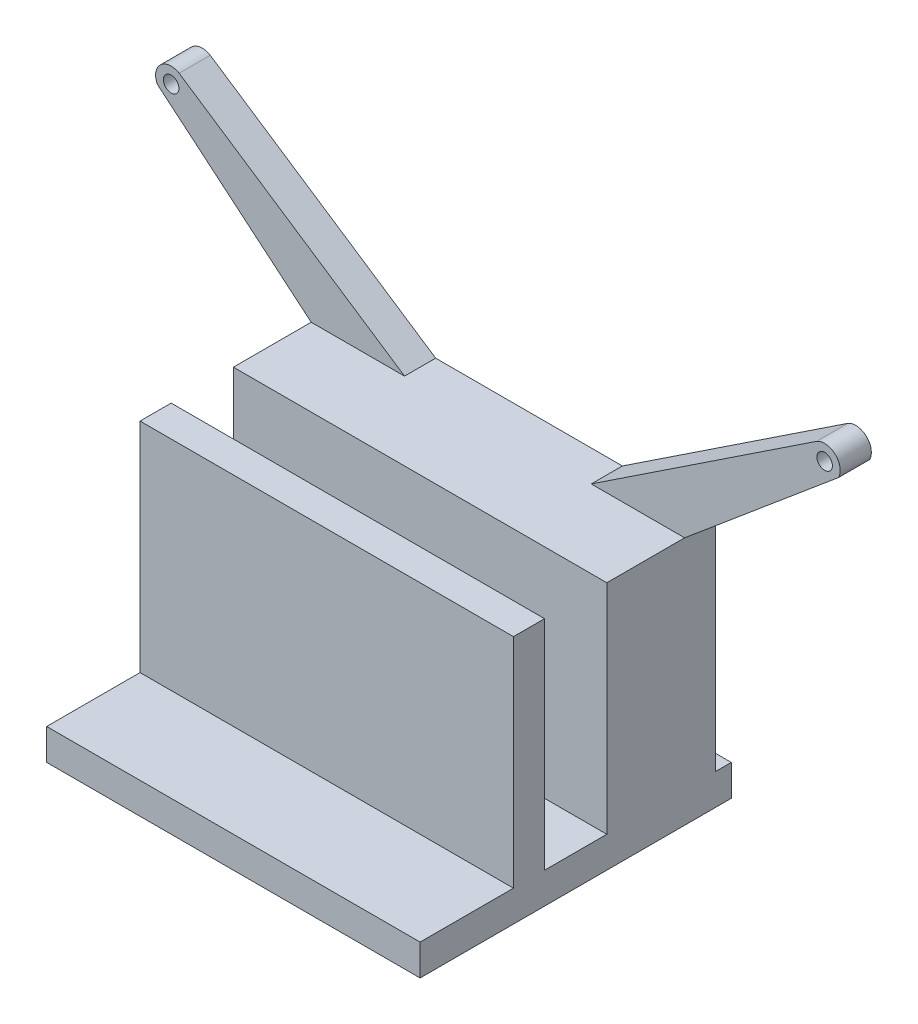
ISO-10303-21;
HEADER;
FILE_DESCRIPTION(('STEP AP214'),'2;1');
FILE_NAME('part.step','',(''),(''),'','','');
FILE_SCHEMA(('AUTOMOTIVE_DESIGN { 1 0 10303 214 1 1 1 1 }'));
ENDSEC;
DATA;
#1=APPLICATION_CONTEXT('core data for automotive mechanical design processes');
#2=APPLICATION_PROTOCOL_DEFINITION('international standard','automotive_design',2000,#1);
#3=PRODUCT_CONTEXT('',#1,'mechanical');
#4=PRODUCT('Part','Part','',(#3));
#5=PRODUCT_RELATED_PRODUCT_CATEGORY('part','',(#4));
#6=PRODUCT_DEFINITION_FORMATION('','',#4);
#7=PRODUCT_DEFINITION_CONTEXT('part definition',#1,'design');
#8=PRODUCT_DEFINITION('design','',#6,#7);
#9=PRODUCT_DEFINITION_SHAPE('','',#8);
#10=(LENGTH_UNIT() NAMED_UNIT(*) SI_UNIT(.MILLI.,.METRE.));
#11=(NAMED_UNIT(*) PLANE_ANGLE_UNIT() SI_UNIT($,.RADIAN.));
#12=(NAMED_UNIT(*) SI_UNIT($,.STERADIAN.) SOLID_ANGLE_UNIT());
#13=UNCERTAINTY_MEASURE_WITH_UNIT(LENGTH_MEASURE(1.E-05),#10,'distance_accuracy_value','');
#14=(GEOMETRIC_REPRESENTATION_CONTEXT(3) GLOBAL_UNCERTAINTY_ASSIGNED_CONTEXT((#13)) GLOBAL_UNIT_ASSIGNED_CONTEXT((#10,
#11,#12)) REPRESENTATION_CONTEXT('',''));
#15=CARTESIAN_POINT('',(0.,0.,0.));
#16=DIRECTION('',(0.,0.,1.));
#17=DIRECTION('',(1.,0.,0.));
#18=AXIS2_PLACEMENT_3D('',#15,#16,#17);
#19=CARTESIAN_POINT('',(0.,-30.,100.));
#20=DIRECTION('',(0.,-1.,0.));
#21=DIRECTION('',(0.,0.,-1.));
#22=AXIS2_PLACEMENT_3D('',#19,#20,#21);
#23=PLANE('',#22);
#24=DIRECTION('',(-1.,0.,0.));
#25=VECTOR('',#24,1.);
#26=CARTESIAN_POINT('',(0.,-30.,60.));
#27=LINE('',#26,#25);
#28=CARTESIAN_POINT('',(60.,-30.,60.));
#29=VERTEX_POINT('',#28);
#30=CARTESIAN_POINT('',(-60.,-30.,60.));
#31=VERTEX_POINT('',#30);
#32=EDGE_CURVE('E60',#29,#31,#27,.T.);
#33=ORIENTED_EDGE('',*,*,#32,.F.);
#34=DIRECTION('',(0.,0.,-1.));
#35=VECTOR('',#34,1.);
#36=CARTESIAN_POINT('',(60.,-30.,100.));
#37=LINE('',#36,#35);
#38=CARTESIAN_POINT('',(60.,-30.,40.));
#39=VERTEX_POINT('',#38);
#40=EDGE_CURVE('E47',#29,#39,#37,.T.);
#41=ORIENTED_EDGE('',*,*,#40,.T.);
#42=DIRECTION('',(-1.,0.,0.));
#43=VECTOR('',#42,1.);
#44=CARTESIAN_POINT('',(0.,-30.,40.));
#45=LINE('',#44,#43);
#46=CARTESIAN_POINT('',(-60.,-30.,40.));
#47=VERTEX_POINT('',#46);
#48=EDGE_CURVE('E555',#39,#47,#45,.T.);
#49=ORIENTED_EDGE('',*,*,#48,.T.);
#50=DIRECTION('',(0.,0.,-1.));
#51=VECTOR('',#50,1.);
#52=CARTESIAN_POINT('',(-60.,-30.,100.));
#53=LINE('',#52,#51);
#54=EDGE_CURVE('E228',#31,#47,#53,.T.);
#55=ORIENTED_EDGE('',*,*,#54,.F.);
#56=EDGE_LOOP('',(#33,#41,#49,#55));
#57=FACE_BOUND('',#56,.T.);
#58=ADVANCED_FACE('F41',(#57),#23,.F.);
#59=CARTESIAN_POINT('',(0.,40.,40.));
#60=DIRECTION('',(0.,-1.,0.));
#61=DIRECTION('',(1.,0.,0.));
#62=AXIS2_PLACEMENT_3D('',#59,#60,#61);
#63=PLANE('',#62);
#64=DIRECTION('',(0.,0.,-1.));
#65=VECTOR('',#64,1.);
#66=CARTESIAN_POINT('',(-30.,40.,15.));
#67=LINE('',#66,#65);
#68=CARTESIAN_POINT('',(-30.,40.,15.));
#69=VERTEX_POINT('',#68);
#70=CARTESIAN_POINT('',(-30.,40.,5.));
#71=VERTEX_POINT('',#70);
#72=EDGE_CURVE('E63',#69,#71,#67,.T.);
#73=ORIENTED_EDGE('',*,*,#72,.F.);
#74=DIRECTION('',(-1.,0.,0.));
#75=VECTOR('',#74,1.);
#76=CARTESIAN_POINT('',(0.,40.,15.));
#77=LINE('',#76,#75);
#78=CARTESIAN_POINT('',(-60.,40.,15.));
#79=VERTEX_POINT('',#78);
#80=EDGE_CURVE('E620',#69,#79,#77,.T.);
#81=ORIENTED_EDGE('',*,*,#80,.T.);
#82=DIRECTION('',(0.,0.,-1.));
#83=VECTOR('',#82,1.);
#84=CARTESIAN_POINT('',(-60.,40.,40.));
#85=LINE('',#84,#83);
#86=CARTESIAN_POINT('',(-60.,40.,40.));
#87=VERTEX_POINT('',#86);
#88=EDGE_CURVE('E264',#87,#79,#85,.T.);
#89=ORIENTED_EDGE('',*,*,#88,.F.);
#90=DIRECTION('',(-1.,0.,0.));
#91=VECTOR('',#90,1.);
#92=CARTESIAN_POINT('',(0.,40.,40.));
#93=LINE('',#92,#91);
#94=CARTESIAN_POINT('',(60.,40.,40.));
#95=VERTEX_POINT('',#94);
#96=EDGE_CURVE('E271',#95,#87,#93,.T.);
#97=ORIENTED_EDGE('',*,*,#96,.F.);
#98=DIRECTION('',(0.,0.,-1.));
#99=VECTOR('',#98,1.);
#100=CARTESIAN_POINT('',(60.,40.,40.));
#101=LINE('',#100,#99);
#102=CARTESIAN_POINT('',(60.,40.,15.));
#103=VERTEX_POINT('',#102);
#104=EDGE_CURVE('E213',#95,#103,#101,.T.);
#105=ORIENTED_EDGE('',*,*,#104,.T.);
#106=DIRECTION('',(-1.,0.,0.));
#107=VECTOR('',#106,1.);
#108=CARTESIAN_POINT('',(0.,40.,15.));
#109=LINE('',#108,#107);
#110=CARTESIAN_POINT('',(30.,40.,15.));
#111=VERTEX_POINT('',#110);
#112=EDGE_CURVE('E569',#103,#111,#109,.T.);
#113=ORIENTED_EDGE('',*,*,#112,.T.);
#114=DIRECTION('',(0.,0.,-1.));
#115=VECTOR('',#114,1.);
#116=CARTESIAN_POINT('',(30.,40.,15.));
#117=LINE('',#116,#115);
#118=CARTESIAN_POINT('',(30.,40.,5.));
#119=VERTEX_POINT('',#118);
#120=EDGE_CURVE('E564',#111,#119,#117,.T.);
#121=ORIENTED_EDGE('',*,*,#120,.T.);
#122=DIRECTION('',(-1.,0.,0.));
#123=VECTOR('',#122,1.);
#124=CARTESIAN_POINT('',(0.,40.,5.));
#125=LINE('',#124,#123);
#126=EDGE_CURVE('E258',#119,#71,#125,.T.);
#127=ORIENTED_EDGE('',*,*,#126,.T.);
#128=EDGE_LOOP('',(#73,#81,#89,#97,#105,#113,#121,#127));
#129=FACE_BOUND('',#128,.T.);
#130=ADVANCED_FACE('F308',(#129),#63,.F.);
#131=DIRECTION('',(-1.,0.,0.));
#132=VECTOR('',#131,1.);
#133=CARTESIAN_POINT('',(0.,-30.,5.));
#134=LINE('',#133,#132);
#135=CARTESIAN_POINT('',(60.,-30.,5.));
#136=VERTEX_POINT('',#135);
#137=CARTESIAN_POINT('',(-60.,-30.,5.));
#138=VERTEX_POINT('',#137);
#139=EDGE_CURVE('E260',#136,#138,#134,.T.);
#140=ORIENTED_EDGE('',*,*,#139,.F.);
#141=CARTESIAN_POINT('',(60.,-30.,0.));
#142=VERTEX_POINT('',#141);
#143=EDGE_CURVE('E49',#136,#142,#37,.T.);
#144=ORIENTED_EDGE('',*,*,#143,.T.);
#145=DIRECTION('',(-1.,0.,0.));
#146=VECTOR('',#145,1.);
#147=CARTESIAN_POINT('',(0.,-30.,0.));
#148=LINE('',#147,#146);
#149=CARTESIAN_POINT('',(-60.,-30.,0.));
#150=VERTEX_POINT('',#149);
#151=EDGE_CURVE('E225',#142,#150,#148,.T.);
#152=ORIENTED_EDGE('',*,*,#151,.T.);
#153=EDGE_CURVE('E226',#138,#150,#53,.T.);
#154=ORIENTED_EDGE('',*,*,#153,.F.);
#155=EDGE_LOOP('',(#140,#144,#152,#154));
#156=FACE_BOUND('',#155,.T.);
#157=ADVANCED_FACE('F244',(#156),#23,.F.);
#158=CARTESIAN_POINT('',(60.,0.,100.));
#159=DIRECTION('',(1.,0.,0.));
#160=DIRECTION('',(0.,1.,0.));
#161=AXIS2_PLACEMENT_3D('',#158,#159,#160);
#162=PLANE('',#161);
#163=DIRECTION('',(0.,-1.,0.));
#164=VECTOR('',#163,1.);
#165=CARTESIAN_POINT('',(60.,0.,0.));
#166=LINE('',#165,#164);
#167=CARTESIAN_POINT('',(60.,-40.,0.));
#168=VERTEX_POINT('',#167);
#169=EDGE_CURVE('E218',#142,#168,#166,.T.);
#170=ORIENTED_EDGE('',*,*,#169,.F.);
#171=ORIENTED_EDGE('',*,*,#143,.F.);
#172=DIRECTION('',(0.,-1.,0.));
#173=VECTOR('',#172,1.);
#174=CARTESIAN_POINT('',(60.,0.,5.));
#175=LINE('',#174,#173);
#176=CARTESIAN_POINT('',(60.,40.,5.));
#177=VERTEX_POINT('',#176);
#178=EDGE_CURVE('E253',#177,#136,#175,.T.);
#179=ORIENTED_EDGE('',*,*,#178,.F.);
#180=DIRECTION('',(0.,0.,-1.));
#181=VECTOR('',#180,1.);
#182=CARTESIAN_POINT('',(60.,40.,15.));
#183=LINE('',#182,#181);
#184=EDGE_CURVE('E252',#103,#177,#183,.T.);
#185=ORIENTED_EDGE('',*,*,#184,.F.);
#186=ORIENTED_EDGE('',*,*,#104,.F.);
#187=DIRECTION('',(0.,-1.,0.));
#188=VECTOR('',#187,1.);
#189=CARTESIAN_POINT('',(60.,0.,40.));
#190=LINE('',#189,#188);
#191=EDGE_CURVE('E280',#95,#39,#190,.T.);
#192=ORIENTED_EDGE('',*,*,#191,.T.);
#193=ORIENTED_EDGE('',*,*,#40,.F.);
#194=DIRECTION('',(0.,-1.,0.));
#195=VECTOR('',#194,1.);
#196=CARTESIAN_POINT('',(60.,0.,60.));
#197=LINE('',#196,#195);
#198=CARTESIAN_POINT('',(60.,40.,60.));
#199=VERTEX_POINT('',#198);
#200=EDGE_CURVE('E632',#199,#29,#197,.T.);
#201=ORIENTED_EDGE('',*,*,#200,.F.);
#202=DIRECTION('',(0.,0.,-1.));
#203=VECTOR('',#202,1.);
#204=CARTESIAN_POINT('',(60.,40.,70.));
#205=LINE('',#204,#203);
#206=CARTESIAN_POINT('',(60.,40.,70.));
#207=VERTEX_POINT('',#206);
#208=EDGE_CURVE('E188',#207,#199,#205,.T.);
#209=ORIENTED_EDGE('',*,*,#208,.F.);
#210=DIRECTION('',(0.,-1.,0.));
#211=VECTOR('',#210,1.);
#212=CARTESIAN_POINT('',(60.,0.,70.));
#213=LINE('',#212,#211);
#214=CARTESIAN_POINT('',(60.,-30.,70.));
#215=VERTEX_POINT('',#214);
#216=EDGE_CURVE('E180',#207,#215,#213,.T.);
#217=ORIENTED_EDGE('',*,*,#216,.T.);
#218=CARTESIAN_POINT('',(60.,-30.,100.));
#219=VERTEX_POINT('',#218);
#220=EDGE_CURVE('E11',#219,#215,#37,.T.);
#221=ORIENTED_EDGE('',*,*,#220,.F.);
#222=DIRECTION('',(0.,-1.,0.));
#223=VECTOR('',#222,1.);
#224=CARTESIAN_POINT('',(60.,0.,100.));
#225=LINE('',#224,#223);
#226=CARTESIAN_POINT('',(60.,-40.,100.));
#227=VERTEX_POINT('',#226);
#228=EDGE_CURVE('E203',#219,#227,#225,.T.);
#229=ORIENTED_EDGE('',*,*,#228,.T.);
#230=DIRECTION('',(0.,0.,-1.));
#231=VECTOR('',#230,1.);
#232=CARTESIAN_POINT('',(60.,-40.,100.));
#233=LINE('',#232,#231);
#234=EDGE_CURVE('E217',#227,#168,#233,.T.);
#235=ORIENTED_EDGE('',*,*,#234,.T.);
#236=EDGE_LOOP('',(#170,#171,#179,#185,#186,#192,#193,#201,#209,#217,#221,#229,#235));
#237=FACE_BOUND('',#236,.T.);
#238=ADVANCED_FACE('F43',(#237),#162,.T.);
#239=ORIENTED_EDGE('',*,*,#220,.T.);
#240=DIRECTION('',(-1.,0.,0.));
#241=VECTOR('',#240,1.);
#242=CARTESIAN_POINT('',(0.,-30.,70.));
#243=LINE('',#242,#241);
#244=CARTESIAN_POINT('',(-60.,-30.,70.));
#245=VERTEX_POINT('',#244);
#246=EDGE_CURVE('E171',#215,#245,#243,.T.);
#247=ORIENTED_EDGE('',*,*,#246,.T.);
#248=CARTESIAN_POINT('',(-60.,-30.,100.));
#249=VERTEX_POINT('',#248);
#250=EDGE_CURVE('E197',#249,#245,#53,.T.);
#251=ORIENTED_EDGE('',*,*,#250,.F.);
#252=DIRECTION('',(-1.,0.,0.));
#253=VECTOR('',#252,1.);
#254=CARTESIAN_POINT('',(0.,-30.,100.));
#255=LINE('',#254,#253);
#256=EDGE_CURVE('E194',#219,#249,#255,.T.);
#257=ORIENTED_EDGE('',*,*,#256,.F.);
#258=EDGE_LOOP('',(#239,#247,#251,#257));
#259=FACE_BOUND('',#258,.T.);
#260=ADVANCED_FACE('F192',(#259),#23,.F.);
#261=CARTESIAN_POINT('',(-60.,0.,100.));
#262=DIRECTION('',(1.,0.,0.));
#263=DIRECTION('',(0.,1.,0.));
#264=AXIS2_PLACEMENT_3D('',#261,#262,#263);
#265=PLANE('',#264);
#266=DIRECTION('',(0.,-1.,0.));
#267=VECTOR('',#266,1.);
#268=CARTESIAN_POINT('',(-60.,0.,0.));
#269=LINE('',#268,#267);
#270=CARTESIAN_POINT('',(-60.,-40.,0.));
#271=VERTEX_POINT('',#270);
#272=EDGE_CURVE('E209',#150,#271,#269,.T.);
#273=ORIENTED_EDGE('',*,*,#272,.T.);
#274=DIRECTION('',(0.,0.,-1.));
#275=VECTOR('',#274,1.);
#276=CARTESIAN_POINT('',(-60.,-40.,100.));
#277=LINE('',#276,#275);
#278=CARTESIAN_POINT('',(-60.,-40.,100.));
#279=VERTEX_POINT('',#278);
#280=EDGE_CURVE('E230',#279,#271,#277,.T.);
#281=ORIENTED_EDGE('',*,*,#280,.F.);
#282=DIRECTION('',(0.,-1.,0.));
#283=VECTOR('',#282,1.);
#284=CARTESIAN_POINT('',(-60.,0.,100.));
#285=LINE('',#284,#283);
#286=EDGE_CURVE('E199',#249,#279,#285,.T.);
#287=ORIENTED_EDGE('',*,*,#286,.F.);
#288=ORIENTED_EDGE('',*,*,#250,.T.);
#289=DIRECTION('',(0.,-1.,0.));
#290=VECTOR('',#289,1.);
#291=CARTESIAN_POINT('',(-60.,0.,70.));
#292=LINE('',#291,#290);
#293=CARTESIAN_POINT('',(-60.,40.,70.));
#294=VERTEX_POINT('',#293);
#295=EDGE_CURVE('E177',#294,#245,#292,.T.);
#296=ORIENTED_EDGE('',*,*,#295,.F.);
#297=DIRECTION('',(0.,0.,-1.));
#298=VECTOR('',#297,1.);
#299=CARTESIAN_POINT('',(-60.,40.,70.));
#300=LINE('',#299,#298);
#301=CARTESIAN_POINT('',(-60.,40.,60.));
#302=VERTEX_POINT('',#301);
#303=EDGE_CURVE('E630',#294,#302,#300,.T.);
#304=ORIENTED_EDGE('',*,*,#303,.T.);
#305=DIRECTION('',(0.,-1.,0.));
#306=VECTOR('',#305,1.);
#307=CARTESIAN_POINT('',(-60.,0.,60.));
#308=LINE('',#307,#306);
#309=EDGE_CURVE('E181',#302,#31,#308,.T.);
#310=ORIENTED_EDGE('',*,*,#309,.T.);
#311=ORIENTED_EDGE('',*,*,#54,.T.);
#312=DIRECTION('',(0.,-1.,0.));
#313=VECTOR('',#312,1.);
#314=CARTESIAN_POINT('',(-60.,0.,40.));
#315=LINE('',#314,#313);
#316=EDGE_CURVE('E270',#87,#47,#315,.T.);
#317=ORIENTED_EDGE('',*,*,#316,.F.);
#318=ORIENTED_EDGE('',*,*,#88,.T.);
#319=DIRECTION('',(0.,0.,-1.));
#320=VECTOR('',#319,1.);
#321=CARTESIAN_POINT('',(-60.,40.,15.));
#322=LINE('',#321,#320);
#323=CARTESIAN_POINT('',(-60.,40.,5.));
#324=VERTEX_POINT('',#323);
#325=EDGE_CURVE('E600',#79,#324,#322,.T.);
#326=ORIENTED_EDGE('',*,*,#325,.T.);
#327=DIRECTION('',(0.,-1.,0.));
#328=VECTOR('',#327,1.);
#329=CARTESIAN_POINT('',(-60.,0.,5.));
#330=LINE('',#329,#328);
#331=EDGE_CURVE('E240',#324,#138,#330,.T.);
#332=ORIENTED_EDGE('',*,*,#331,.T.);
#333=ORIENTED_EDGE('',*,*,#153,.T.);
#334=EDGE_LOOP('',(#273,#281,#287,#288,#296,#304,#310,#311,#317,#318,#326,#332,#333));
#335=FACE_BOUND('',#334,.T.);
#336=ADVANCED_FACE('F231',(#335),#265,.F.);
#337=CARTESIAN_POINT('',(0.,-40.,100.));
#338=DIRECTION('',(0.,-1.,0.));
#339=DIRECTION('',(0.,0.,-1.));
#340=AXIS2_PLACEMENT_3D('',#337,#338,#339);
#341=PLANE('',#340);
#342=DIRECTION('',(-1.,0.,0.));
#343=VECTOR('',#342,1.);
#344=CARTESIAN_POINT('',(0.,-40.,0.));
#345=LINE('',#344,#343);
#346=EDGE_CURVE('E210',#168,#271,#345,.T.);
#347=ORIENTED_EDGE('',*,*,#346,.F.);
#348=ORIENTED_EDGE('',*,*,#234,.F.);
#349=DIRECTION('',(-1.,0.,0.));
#350=VECTOR('',#349,1.);
#351=CARTESIAN_POINT('',(0.,-40.,100.));
#352=LINE('',#351,#350);
#353=EDGE_CURVE('E206',#227,#279,#352,.T.);
#354=ORIENTED_EDGE('',*,*,#353,.T.);
#355=ORIENTED_EDGE('',*,*,#280,.T.);
#356=EDGE_LOOP('',(#347,#348,#354,#355));
#357=FACE_BOUND('',#356,.T.);
#358=ADVANCED_FACE('F246',(#357),#341,.T.);
#359=CARTESIAN_POINT('',(0.,0.,100.));
#360=DIRECTION('',(0.,0.,1.));
#361=DIRECTION('',(1.,0.,0.));
#362=AXIS2_PLACEMENT_3D('',#359,#360,#361);
#363=PLANE('',#362);
#364=ORIENTED_EDGE('',*,*,#228,.F.);
#365=ORIENTED_EDGE('',*,*,#256,.T.);
#366=ORIENTED_EDGE('',*,*,#286,.T.);
#367=ORIENTED_EDGE('',*,*,#353,.F.);
#368=EDGE_LOOP('',(#364,#365,#366,#367));
#369=FACE_BOUND('',#368,.T.);
#370=ADVANCED_FACE('F204',(#369),#363,.T.);
#371=CARTESIAN_POINT('',(0.,0.,0.));
#372=DIRECTION('',(0.,0.,1.));
#373=DIRECTION('',(1.,0.,0.));
#374=AXIS2_PLACEMENT_3D('',#371,#372,#373);
#375=PLANE('',#374);
#376=ORIENTED_EDGE('',*,*,#169,.T.);
#377=ORIENTED_EDGE('',*,*,#346,.T.);
#378=ORIENTED_EDGE('',*,*,#272,.F.);
#379=ORIENTED_EDGE('',*,*,#151,.F.);
#380=EDGE_LOOP('',(#376,#377,#378,#379));
#381=FACE_BOUND('',#380,.T.);
#382=ADVANCED_FACE('F243',(#381),#375,.F.);
#383=CARTESIAN_POINT('',(-30.,0.,40.));
#384=DIRECTION('',(0.,0.,-1.));
#385=DIRECTION('',(-1.,0.,0.));
#386=AXIS2_PLACEMENT_3D('',#383,#384,#385);
#387=CYLINDRICAL_SURFACE('',#386,4.);
#388=CARTESIAN_POINT('',(-30.,0.,40.));
#389=DIRECTION('',(0.,0.,1.));
#390=DIRECTION('',(1.,0.,0.));
#391=AXIS2_PLACEMENT_3D('',#388,#389,#390);
#392=CIRCLE('',#391,4.);
#393=CARTESIAN_POINT('',(-26.,0.,40.));
#394=VERTEX_POINT('',#393);
#395=EDGE_CURVE('E549',#394,#394,#392,.T.);
#396=ORIENTED_EDGE('',*,*,#395,.T.);
#397=EDGE_LOOP('',(#396));
#398=FACE_BOUND('',#397,.T.);
#399=CARTESIAN_POINT('',(-30.,0.,5.));
#400=DIRECTION('',(0.,0.,1.));
#401=DIRECTION('',(1.,0.,0.));
#402=AXIS2_PLACEMENT_3D('',#399,#400,#401);
#403=CIRCLE('',#402,4.);
#404=CARTESIAN_POINT('',(-26.,0.,5.));
#405=VERTEX_POINT('',#404);
#406=EDGE_CURVE('E257',#405,#405,#403,.T.);
#407=ORIENTED_EDGE('',*,*,#406,.F.);
#408=EDGE_LOOP('',(#407));
#409=FACE_BOUND('',#408,.T.);
#410=ADVANCED_FACE('F287',(#398,#409),#387,.F.);
#411=CARTESIAN_POINT('',(30.,0.,40.));
#412=DIRECTION('',(0.,0.,-1.));
#413=DIRECTION('',(-1.,0.,0.));
#414=AXIS2_PLACEMENT_3D('',#411,#412,#413);
#415=CYLINDRICAL_SURFACE('',#414,4.);
#416=CARTESIAN_POINT('',(30.,0.,40.));
#417=DIRECTION('',(0.,0.,1.));
#418=DIRECTION('',(1.,0.,0.));
#419=AXIS2_PLACEMENT_3D('',#416,#417,#418);
#420=CIRCLE('',#419,4.);
#421=CARTESIAN_POINT('',(34.,0.,40.));
#422=VERTEX_POINT('',#421);
#423=EDGE_CURVE('E262',#422,#422,#420,.T.);
#424=ORIENTED_EDGE('',*,*,#423,.T.);
#425=EDGE_LOOP('',(#424));
#426=FACE_BOUND('',#425,.T.);
#427=CARTESIAN_POINT('',(30.,0.,5.));
#428=DIRECTION('',(0.,0.,1.));
#429=DIRECTION('',(1.,0.,0.));
#430=AXIS2_PLACEMENT_3D('',#427,#428,#429);
#431=CIRCLE('',#430,4.);
#432=CARTESIAN_POINT('',(34.,0.,5.));
#433=VERTEX_POINT('',#432);
#434=EDGE_CURVE('E282',#433,#433,#431,.T.);
#435=ORIENTED_EDGE('',*,*,#434,.F.);
#436=EDGE_LOOP('',(#435));
#437=FACE_BOUND('',#436,.T.);
#438=ADVANCED_FACE('F292',(#426,#437),#415,.F.);
#439=CARTESIAN_POINT('',(0.,0.,40.));
#440=DIRECTION('',(0.,0.,1.));
#441=DIRECTION('',(1.,0.,0.));
#442=AXIS2_PLACEMENT_3D('',#439,#440,#441);
#443=PLANE('',#442);
#444=ORIENTED_EDGE('',*,*,#423,.F.);
#445=EDGE_LOOP('',(#444));
#446=FACE_BOUND('',#445,.T.);
#447=ORIENTED_EDGE('',*,*,#395,.F.);
#448=EDGE_LOOP('',(#447));
#449=FACE_BOUND('',#448,.T.);
#450=ORIENTED_EDGE('',*,*,#48,.F.);
#451=ORIENTED_EDGE('',*,*,#191,.F.);
#452=ORIENTED_EDGE('',*,*,#96,.T.);
#453=ORIENTED_EDGE('',*,*,#316,.T.);
#454=EDGE_LOOP('',(#450,#451,#452,#453));
#455=FACE_BOUND('',#454,.T.);
#456=ADVANCED_FACE('F300',(#446,#449,#455),#443,.T.);
#457=CARTESIAN_POINT('',(0.,0.,5.));
#458=DIRECTION('',(0.,0.,1.));
#459=DIRECTION('',(1.,0.,0.));
#460=AXIS2_PLACEMENT_3D('',#457,#458,#459);
#461=PLANE('',#460);
#462=ORIENTED_EDGE('',*,*,#434,.T.);
#463=EDGE_LOOP('',(#462));
#464=FACE_BOUND('',#463,.T.);
#465=ORIENTED_EDGE('',*,*,#406,.T.);
#466=EDGE_LOOP('',(#465));
#467=FACE_BOUND('',#466,.T.);
#468=ORIENTED_EDGE('',*,*,#139,.T.);
#469=ORIENTED_EDGE('',*,*,#331,.F.);
#470=DIRECTION('',(-0.766044443118975,0.642787609686543,0.));
#471=VECTOR('',#470,1.);
#472=CARTESIAN_POINT('',(-5.09439960974816,-6.07126903702785,5.));
#473=LINE('',#472,#471);
#474=CARTESIAN_POINT('',(-109.439765001314,81.4848885780946,5.));
#475=VERTEX_POINT('',#474);
#476=EDGE_CURVE('E610',#324,#475,#473,.T.);
#477=ORIENTED_EDGE('',*,*,#476,.T.);
#478=CARTESIAN_POINT('',(-105.,83.7845595835005,5.));
#479=DIRECTION('',(0.,0.,1.));
#480=DIRECTION('',(1.,0.,0.));
#481=AXIS2_PLACEMENT_3D('',#478,#479,#480);
#482=CIRCLE('',#481,5.);
#483=CARTESIAN_POINT('',(-102.433113427813,88.0753745789913,5.));
#484=VERTEX_POINT('',#483);
#485=EDGE_CURVE('E608',#475,#484,#482,.F.);
#486=ORIENTED_EDGE('',*,*,#485,.T.);
#487=DIRECTION('',(-0.833181322159972,0.552999895482596,0.));
#488=VECTOR('',#487,1.);
#489=CARTESIAN_POINT('',(9.25570083078775,13.9451691016741,5.));
#490=LINE('',#489,#488);
#491=EDGE_CURVE('E602',#71,#484,#490,.T.);
#492=ORIENTED_EDGE('',*,*,#491,.F.);
#493=ORIENTED_EDGE('',*,*,#126,.F.);
#494=DIRECTION('',(0.833181322159971,0.552999895482596,0.));
#495=VECTOR('',#494,1.);
#496=CARTESIAN_POINT('',(-9.25570083078775,13.9451691016741,5.));
#497=LINE('',#496,#495);
#498=CARTESIAN_POINT('',(102.433113427813,88.0753745789913,5.));
#499=VERTEX_POINT('',#498);
#500=EDGE_CURVE('E568',#119,#499,#497,.T.);
#501=ORIENTED_EDGE('',*,*,#500,.T.);
#502=CARTESIAN_POINT('',(105.,83.7845595835005,5.));
#503=DIRECTION('',(0.,0.,1.));
#504=DIRECTION('',(1.,0.,0.));
#505=AXIS2_PLACEMENT_3D('',#502,#503,#504);
#506=CIRCLE('',#505,5.);
#507=CARTESIAN_POINT('',(109.439765001314,81.4848885780946,5.));
#508=VERTEX_POINT('',#507);
#509=EDGE_CURVE('E571',#508,#499,#506,.T.);
#510=ORIENTED_EDGE('',*,*,#509,.F.);
#511=DIRECTION('',(0.766044443118975,0.642787609686543,0.));
#512=VECTOR('',#511,1.);
#513=CARTESIAN_POINT('',(5.09439960974816,-6.07126903702785,5.));
#514=LINE('',#513,#512);
#515=EDGE_CURVE('E580',#177,#508,#514,.T.);
#516=ORIENTED_EDGE('',*,*,#515,.F.);
#517=ORIENTED_EDGE('',*,*,#178,.T.);
#518=EDGE_LOOP('',(#468,#469,#477,#486,#492,#493,#501,#510,#516,#517));
#519=FACE_BOUND('',#518,.T.);
#520=CARTESIAN_POINT('',(105.,83.7845595835005,5.));
#521=DIRECTION('',(0.,0.,1.));
#522=DIRECTION('',(1.,0.,0.));
#523=AXIS2_PLACEMENT_3D('',#520,#521,#522);
#524=CIRCLE('',#523,2.5);
#525=CARTESIAN_POINT('',(107.5,83.7845595835005,5.));
#526=VERTEX_POINT('',#525);
#527=EDGE_CURVE('E579',#526,#526,#524,.F.);
#528=ORIENTED_EDGE('',*,*,#527,.F.);
#529=EDGE_LOOP('',(#528));
#530=FACE_BOUND('',#529,.T.);
#531=CARTESIAN_POINT('',(-105.,83.7845595835005,5.));
#532=DIRECTION('',(0.,0.,1.));
#533=DIRECTION('',(1.,0.,0.));
#534=AXIS2_PLACEMENT_3D('',#531,#532,#533);
#535=CIRCLE('',#534,2.5);
#536=CARTESIAN_POINT('',(-102.5,83.7845595835005,5.));
#537=VERTEX_POINT('',#536);
#538=EDGE_CURVE('E615',#537,#537,#535,.T.);
#539=ORIENTED_EDGE('',*,*,#538,.T.);
#540=EDGE_LOOP('',(#539));
#541=FACE_BOUND('',#540,.T.);
#542=ADVANCED_FACE('F290',(#464,#467,#519,#530,#541),#461,.F.);
#543=CARTESIAN_POINT('',(5.09439960974816,-6.07126903702785,15.));
#544=DIRECTION('',(-0.642787609686543,0.766044443118975,0.));
#545=DIRECTION('',(-0.766044443118975,-0.642787609686543,0.));
#546=AXIS2_PLACEMENT_3D('',#543,#544,#545);
#547=PLANE('',#546);
#548=ORIENTED_EDGE('',*,*,#515,.T.);
#549=DIRECTION('',(0.,0.,-1.));
#550=VECTOR('',#549,1.);
#551=CARTESIAN_POINT('',(109.439765001314,81.4848885780946,15.));
#552=LINE('',#551,#550);
#553=CARTESIAN_POINT('',(109.439765001314,81.4848885780946,15.));
#554=VERTEX_POINT('',#553);
#555=EDGE_CURVE('E285',#554,#508,#552,.T.);
#556=ORIENTED_EDGE('',*,*,#555,.F.);
#557=DIRECTION('',(0.766044443118975,0.642787609686543,0.));
#558=VECTOR('',#557,1.);
#559=CARTESIAN_POINT('',(5.09439960974816,-6.07126903702785,15.));
#560=LINE('',#559,#558);
#561=EDGE_CURVE('E591',#103,#554,#560,.T.);
#562=ORIENTED_EDGE('',*,*,#561,.F.);
#563=ORIENTED_EDGE('',*,*,#184,.T.);
#564=EDGE_LOOP('',(#548,#556,#562,#563));
#565=FACE_BOUND('',#564,.T.);
#566=ADVANCED_FACE('F396',(#565),#547,.F.);
#567=CARTESIAN_POINT('',(105.,83.7845595835005,15.));
#568=DIRECTION('',(0.,0.,-1.));
#569=DIRECTION('',(-1.,0.,0.));
#570=AXIS2_PLACEMENT_3D('',#567,#568,#569);
#571=CYLINDRICAL_SURFACE('',#570,5.);
#572=ORIENTED_EDGE('',*,*,#509,.T.);
#573=DIRECTION('',(0.,0.,-1.));
#574=VECTOR('',#573,1.);
#575=CARTESIAN_POINT('',(102.433113427813,88.0753745789913,15.));
#576=LINE('',#575,#574);
#577=CARTESIAN_POINT('',(102.433113427813,88.0753745789913,15.));
#578=VERTEX_POINT('',#577);
#579=EDGE_CURVE('E561',#578,#499,#576,.T.);
#580=ORIENTED_EDGE('',*,*,#579,.F.);
#581=CARTESIAN_POINT('',(105.,83.7845595835005,15.));
#582=DIRECTION('',(0.,0.,1.));
#583=DIRECTION('',(1.,0.,0.));
#584=AXIS2_PLACEMENT_3D('',#581,#582,#583);
#585=CIRCLE('',#584,5.);
#586=EDGE_CURVE('E589',#554,#578,#585,.T.);
#587=ORIENTED_EDGE('',*,*,#586,.F.);
#588=ORIENTED_EDGE('',*,*,#555,.T.);
#589=EDGE_LOOP('',(#572,#580,#587,#588));
#590=FACE_BOUND('',#589,.T.);
#591=ADVANCED_FACE('F391',(#590),#571,.T.);
#592=CARTESIAN_POINT('',(-9.25570083078775,13.9451691016741,15.));
#593=DIRECTION('',(-0.552999895482596,0.833181322159971,0.));
#594=DIRECTION('',(-0.833181322159971,-0.552999895482596,0.));
#595=AXIS2_PLACEMENT_3D('',#592,#593,#594);
#596=PLANE('',#595);
#597=ORIENTED_EDGE('',*,*,#500,.F.);
#598=ORIENTED_EDGE('',*,*,#120,.F.);
#599=DIRECTION('',(0.833181322159971,0.552999895482596,0.));
#600=VECTOR('',#599,1.);
#601=CARTESIAN_POINT('',(-9.25570083078775,13.9451691016741,15.));
#602=LINE('',#601,#600);
#603=EDGE_CURVE('E588',#111,#578,#602,.T.);
#604=ORIENTED_EDGE('',*,*,#603,.T.);
#605=ORIENTED_EDGE('',*,*,#579,.T.);
#606=EDGE_LOOP('',(#597,#598,#604,#605));
#607=FACE_BOUND('',#606,.T.);
#608=ADVANCED_FACE('F392',(#607),#596,.T.);
#609=CARTESIAN_POINT('',(105.,83.7845595835005,15.));
#610=DIRECTION('',(0.,0.,-1.));
#611=DIRECTION('',(-1.,0.,0.));
#612=AXIS2_PLACEMENT_3D('',#609,#610,#611);
#613=CYLINDRICAL_SURFACE('',#612,2.5);
#614=CARTESIAN_POINT('',(105.,83.7845595835005,15.));
#615=DIRECTION('',(0.,0.,1.));
#616=DIRECTION('',(1.,0.,0.));
#617=AXIS2_PLACEMENT_3D('',#614,#615,#616);
#618=CIRCLE('',#617,2.5);
#619=CARTESIAN_POINT('',(107.5,83.7845595835005,15.));
#620=VERTEX_POINT('',#619);
#621=EDGE_CURVE('E575',#620,#620,#618,.F.);
#622=ORIENTED_EDGE('',*,*,#621,.F.);
#623=EDGE_LOOP('',(#622));
#624=FACE_BOUND('',#623,.T.);
#625=ORIENTED_EDGE('',*,*,#527,.T.);
#626=EDGE_LOOP('',(#625));
#627=FACE_BOUND('',#626,.T.);
#628=ADVANCED_FACE('F386',(#624,#627),#613,.F.);
#629=CARTESIAN_POINT('',(0.,0.,15.));
#630=DIRECTION('',(0.,0.,1.));
#631=DIRECTION('',(1.,0.,0.));
#632=AXIS2_PLACEMENT_3D('',#629,#630,#631);
#633=PLANE('',#632);
#634=ORIENTED_EDGE('',*,*,#621,.T.);
#635=EDGE_LOOP('',(#634));
#636=FACE_BOUND('',#635,.T.);
#637=ORIENTED_EDGE('',*,*,#561,.T.);
#638=ORIENTED_EDGE('',*,*,#586,.T.);
#639=ORIENTED_EDGE('',*,*,#603,.F.);
#640=ORIENTED_EDGE('',*,*,#112,.F.);
#641=EDGE_LOOP('',(#637,#638,#639,#640));
#642=FACE_BOUND('',#641,.T.);
#643=ADVANCED_FACE('F385',(#636,#642),#633,.T.);
#644=CARTESIAN_POINT('',(-105.,83.7845595835005,15.));
#645=DIRECTION('',(0.,0.,-1.));
#646=DIRECTION('',(-1.,0.,0.));
#647=AXIS2_PLACEMENT_3D('',#644,#645,#646);
#648=CYLINDRICAL_SURFACE('',#647,5.);
#649=ORIENTED_EDGE('',*,*,#485,.F.);
#650=DIRECTION('',(0.,0.,-1.));
#651=VECTOR('',#650,1.);
#652=CARTESIAN_POINT('',(-109.439765001314,81.4848885780946,15.));
#653=LINE('',#652,#651);
#654=CARTESIAN_POINT('',(-109.439765001314,81.4848885780946,15.));
#655=VERTEX_POINT('',#654);
#656=EDGE_CURVE('E581',#655,#475,#653,.T.);
#657=ORIENTED_EDGE('',*,*,#656,.F.);
#658=CARTESIAN_POINT('',(-105.,83.7845595835005,15.));
#659=DIRECTION('',(0.,0.,1.));
#660=DIRECTION('',(1.,0.,0.));
#661=AXIS2_PLACEMENT_3D('',#658,#659,#660);
#662=CIRCLE('',#661,5.);
#663=CARTESIAN_POINT('',(-102.433113427813,88.0753745789913,15.));
#664=VERTEX_POINT('',#663);
#665=EDGE_CURVE('E625',#655,#664,#662,.F.);
#666=ORIENTED_EDGE('',*,*,#665,.T.);
#667=DIRECTION('',(0.,0.,-1.));
#668=VECTOR('',#667,1.);
#669=CARTESIAN_POINT('',(-102.433113427813,88.0753745789913,15.));
#670=LINE('',#669,#668);
#671=EDGE_CURVE('E599',#664,#484,#670,.T.);
#672=ORIENTED_EDGE('',*,*,#671,.T.);
#673=EDGE_LOOP('',(#649,#657,#666,#672));
#674=FACE_BOUND('',#673,.T.);
#675=ADVANCED_FACE('F378',(#674),#648,.T.);
#676=CARTESIAN_POINT('',(-5.09439960974816,-6.07126903702785,15.));
#677=DIRECTION('',(-0.642787609686543,-0.766044443118975,0.));
#678=DIRECTION('',(0.766044443118975,-0.642787609686543,0.));
#679=AXIS2_PLACEMENT_3D('',#676,#677,#678);
#680=PLANE('',#679);
#681=ORIENTED_EDGE('',*,*,#476,.F.);
#682=ORIENTED_EDGE('',*,*,#325,.F.);
#683=DIRECTION('',(-0.766044443118975,0.642787609686543,0.));
#684=VECTOR('',#683,1.);
#685=CARTESIAN_POINT('',(-5.09439960974816,-6.07126903702785,15.));
#686=LINE('',#685,#684);
#687=EDGE_CURVE('E617',#79,#655,#686,.T.);
#688=ORIENTED_EDGE('',*,*,#687,.T.);
#689=ORIENTED_EDGE('',*,*,#656,.T.);
#690=EDGE_LOOP('',(#681,#682,#688,#689));
#691=FACE_BOUND('',#690,.T.);
#692=ADVANCED_FACE('F374',(#691),#680,.T.);
#693=CARTESIAN_POINT('',(-105.,83.7845595835005,15.));
#694=DIRECTION('',(0.,0.,-1.));
#695=DIRECTION('',(-1.,0.,0.));
#696=AXIS2_PLACEMENT_3D('',#693,#694,#695);
#697=CYLINDRICAL_SURFACE('',#696,2.5);
#698=CARTESIAN_POINT('',(-105.,83.7845595835005,15.));
#699=DIRECTION('',(0.,0.,1.));
#700=DIRECTION('',(1.,0.,0.));
#701=AXIS2_PLACEMENT_3D('',#698,#699,#700);
#702=CIRCLE('',#701,2.5);
#703=CARTESIAN_POINT('',(-102.5,83.7845595835005,15.));
#704=VERTEX_POINT('',#703);
#705=EDGE_CURVE('E607',#704,#704,#702,.T.);
#706=ORIENTED_EDGE('',*,*,#705,.T.);
#707=EDGE_LOOP('',(#706));
#708=FACE_BOUND('',#707,.T.);
#709=ORIENTED_EDGE('',*,*,#538,.F.);
#710=EDGE_LOOP('',(#709));
#711=FACE_BOUND('',#710,.T.);
#712=ADVANCED_FACE('F373',(#708,#711),#697,.F.);
#713=CARTESIAN_POINT('',(9.25570083078775,13.9451691016741,15.));
#714=DIRECTION('',(-0.552999895482596,-0.833181322159971,0.));
#715=DIRECTION('',(0.833181322159971,-0.552999895482596,0.));
#716=AXIS2_PLACEMENT_3D('',#713,#714,#715);
#717=PLANE('',#716);
#718=ORIENTED_EDGE('',*,*,#491,.T.);
#719=ORIENTED_EDGE('',*,*,#671,.F.);
#720=DIRECTION('',(-0.833181322159972,0.552999895482596,0.));
#721=VECTOR('',#720,1.);
#722=CARTESIAN_POINT('',(9.25570083078775,13.9451691016741,15.));
#723=LINE('',#722,#721);
#724=EDGE_CURVE('E605',#69,#664,#723,.T.);
#725=ORIENTED_EDGE('',*,*,#724,.F.);
#726=ORIENTED_EDGE('',*,*,#72,.T.);
#727=EDGE_LOOP('',(#718,#719,#725,#726));
#728=FACE_BOUND('',#727,.T.);
#729=ADVANCED_FACE('F369',(#728),#717,.F.);
#730=CARTESIAN_POINT('',(0.,0.,15.));
#731=DIRECTION('',(0.,0.,1.));
#732=DIRECTION('',(1.,0.,0.));
#733=AXIS2_PLACEMENT_3D('',#730,#731,#732);
#734=PLANE('',#733);
#735=ORIENTED_EDGE('',*,*,#705,.F.);
#736=EDGE_LOOP('',(#735));
#737=FACE_BOUND('',#736,.T.);
#738=ORIENTED_EDGE('',*,*,#665,.F.);
#739=ORIENTED_EDGE('',*,*,#687,.F.);
#740=ORIENTED_EDGE('',*,*,#80,.F.);
#741=ORIENTED_EDGE('',*,*,#724,.T.);
#742=EDGE_LOOP('',(#738,#739,#740,#741));
#743=FACE_BOUND('',#742,.T.);
#744=ADVANCED_FACE('F347',(#737,#743),#734,.T.);
#745=CARTESIAN_POINT('',(0.,40.,70.));
#746=DIRECTION('',(0.,-1.,0.));
#747=DIRECTION('',(1.,0.,0.));
#748=AXIS2_PLACEMENT_3D('',#745,#746,#747);
#749=PLANE('',#748);
#750=DIRECTION('',(-1.,0.,0.));
#751=VECTOR('',#750,1.);
#752=CARTESIAN_POINT('',(0.,40.,60.));
#753=LINE('',#752,#751);
#754=EDGE_CURVE('E635',#199,#302,#753,.T.);
#755=ORIENTED_EDGE('',*,*,#754,.T.);
#756=ORIENTED_EDGE('',*,*,#303,.F.);
#757=DIRECTION('',(-1.,0.,0.));
#758=VECTOR('',#757,1.);
#759=CARTESIAN_POINT('',(0.,40.,70.));
#760=LINE('',#759,#758);
#761=EDGE_CURVE('E195',#207,#294,#760,.T.);
#762=ORIENTED_EDGE('',*,*,#761,.F.);
#763=ORIENTED_EDGE('',*,*,#208,.T.);
#764=EDGE_LOOP('',(#755,#756,#762,#763));
#765=FACE_BOUND('',#764,.T.);
#766=ADVANCED_FACE('F343',(#765),#749,.F.);
#767=CARTESIAN_POINT('',(0.,0.,70.));
#768=DIRECTION('',(0.,0.,1.));
#769=DIRECTION('',(1.,0.,0.));
#770=AXIS2_PLACEMENT_3D('',#767,#768,#769);
#771=PLANE('',#770);
#772=ORIENTED_EDGE('',*,*,#246,.F.);
#773=ORIENTED_EDGE('',*,*,#216,.F.);
#774=ORIENTED_EDGE('',*,*,#761,.T.);
#775=ORIENTED_EDGE('',*,*,#295,.T.);
#776=EDGE_LOOP('',(#772,#773,#774,#775));
#777=FACE_BOUND('',#776,.T.);
#778=ADVANCED_FACE('F178',(#777),#771,.T.);
#779=CARTESIAN_POINT('',(0.,0.,60.));
#780=DIRECTION('',(0.,0.,1.));
#781=DIRECTION('',(1.,0.,0.));
#782=AXIS2_PLACEMENT_3D('',#779,#780,#781);
#783=PLANE('',#782);
#784=ORIENTED_EDGE('',*,*,#32,.T.);
#785=ORIENTED_EDGE('',*,*,#309,.F.);
#786=ORIENTED_EDGE('',*,*,#754,.F.);
#787=ORIENTED_EDGE('',*,*,#200,.T.);
#788=EDGE_LOOP('',(#784,#785,#786,#787));
#789=FACE_BOUND('',#788,.T.);
#790=ADVANCED_FACE('F358',(#789),#783,.F.);
#791=CLOSED_SHELL('',(#58,#130,#157,#238,#260,#336,#358,#370,#382,#410,#438,#456,#542,#566,#591,
#608,#628,#643,#675,#692,#712,#729,#744,#766,#778,#790));
#792=MANIFOLD_SOLID_BREP('B2',#791);
#793=ADVANCED_BREP_SHAPE_REPRESENTATION('',(#18,#792),#14);
#794=SHAPE_DEFINITION_REPRESENTATION(#9,#793);
ENDSEC;
END-ISO-10303-21;
